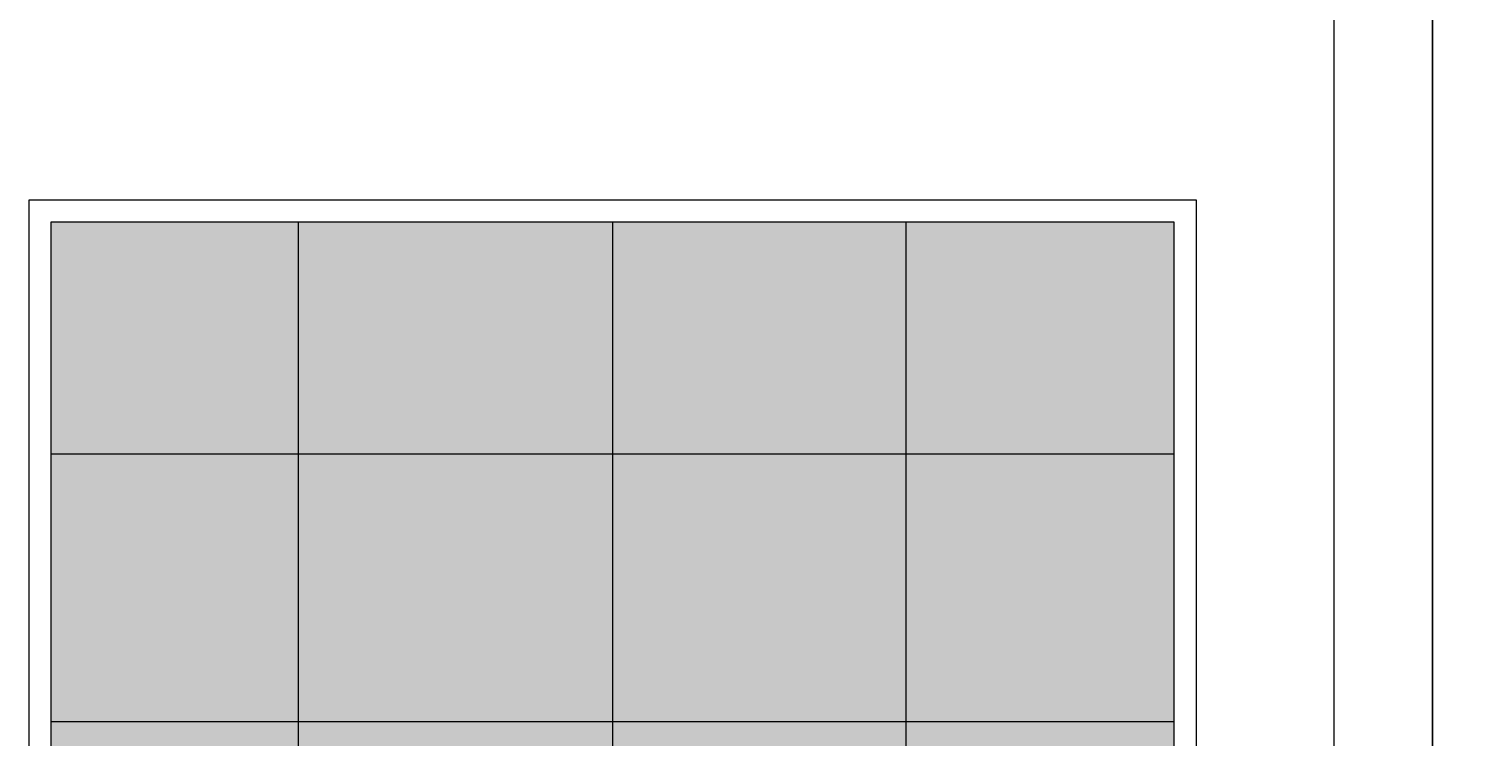
# Model space of a CAD drawing. Units: inches. Extents: x -26 to 776, y -22 to 650.
# Tile 10 of 62: x 92 to 222, y 223 to 287. Entities that reach past the tile are written whole.
import ezdxf

# ---------------------------------------------------------------- set-up
doc = ezdxf.new("R2010")
doc.units = ezdxf.units.IN
doc.header["$MEASUREMENT"] = 0
for name, color, linetype, lineweight in [('A-ANNO-DIMS', 2, 'Continuous', 18), ('A-GLAZ', 4, 'Continuous', 18), ('A-GLAZ-PATT', 9, 'Continuous', 13), ('A-WALL-TRIM', 7, 'Continuous', 18)]:
    doc.layers.add(name, color=color, linetype=linetype, lineweight=lineweight)
doc.styles.get("Standard").update_dxf_attribs({"font": 'arial.ttf'})
doc.dimstyles.get("Standard").update_dxf_attribs({"dimtxt": 0.5625, "dimasz": 0.18, "dimexe": 0.18, "dimexo": 0.0625, "dimgap": 0.09, "dimtad": 0, "dimtih": 1, "dimtoh": 1, "dimdec": 4, "dimzin": 0, "dimdsep": 46, "dimlunit": 4, "dimtxsty": 'Standard', "dimcen": 0.09, "dimadec": 0, "dimazin": 0, "dimtfac": 1, "dimtdec": 4, "dimtofl": 0, "dimtmove": 0, "dimatfit": 3, "dimfxl": 1, "dimtolj": 1, "dimtzin": 0, "dimarcsym": 0})

# ---------------------------------------------------------------- blocks, each defined once
blk = doc.blocks.new('WIN-ELEV-4X4')
for p, q in [((24.2, 97.34), (24.2, 2)), ((52.51, 97.34), (52.51, 2)), ((78.9, 97.34), (78.9, 2)), ((2, 76.47), (103.02, 76.47)), ((2, 76.47), (103.02, 76.47)), ((2, 52.37), (103.02, 52.37)), ((2, 26.9), (103.02, 26.9))]:
    blk.add_line(p, q)
for points in [[(0, 99.34), (105.02, 99.34), (105.02, 0), (0, 0)], [(2, 97.34), (103.02, 97.34), (103.02, 2), (2, 2)]]:
    blk.add_lwpolyline(points, close=True)
blk = doc.blocks.new('*D14')
at = {"layer": 'A-ANNO-DIMS', "color": 0, "lineweight": -2, "transparency": 16777216}
for p, q in [((191.62, 613.27), (-25.48, 613.27)), ((-25.3, 613.09), (-25.3, 314.75)), ((-25.3, 15.66), (-25.3, 314)), ((11.04, 15.48), (-25.48, 15.48))]:
    blk.add_line(p, q, dxfattribs=at)
at = {"layer": 'A-ANNO-DIMS', "color": 0, "transparency": 16777216}
for points in [[(-25.33, 613.09), (-25.27, 613.09), (-25.3, 613.27)], [(-25.33, 15.66), (-25.27, 15.66), (-25.3, 15.48)]]:
    blk.add_solid(points, dxfattribs=at)
at = {"layer": 'Defpoints', "color": 0, "transparency": 16777216}
for p in [(-25.3, 613.27), (191.68, 613.27), (11.11, 15.48)]:
    blk.add_point(p, dxfattribs=at)
at = {"layer": 'A-ANNO-DIMS', "color": 0, "transparency": 16777216, "insert": (-25.3, 314.38), "char_height": 0.562, "attachment_point": 5}
blk.add_mtext('\\A1;597.8', dxfattribs=at)
blk = doc.blocks.new('*D22')
at = {"layer": 'A-ANNO-DIMS', "color": 0, "lineweight": -2, "transparency": 16777216}
for p, q in [((22.89, 15.33), (22.89, 649.86)), ((23.07, 649.68), (119.19, 649.68)), ((217.77, 649.68), (121.65, 649.68)), ((217.95, 15.54), (217.95, 649.86))]:
    blk.add_line(p, q, dxfattribs=at)
at = {"layer": 'A-ANNO-DIMS', "color": 0, "transparency": 16777216}
for points in [[(23.07, 649.71), (23.07, 649.65), (22.89, 649.68)], [(217.77, 649.71), (217.77, 649.65), (217.95, 649.68)]]:
    blk.add_solid(points, dxfattribs=at)
at = {"layer": 'Defpoints', "color": 0, "transparency": 16777216}
for p in [(217.95, 649.68), (22.89, 15.27), (217.95, 15.48)]:
    blk.add_point(p, dxfattribs=at)
at = {"layer": 'A-ANNO-DIMS', "color": 0, "transparency": 16777216, "insert": (120.42, 649.68), "char_height": 0.562, "attachment_point": 5}
blk.add_mtext('\\A1;195.06', dxfattribs=at)

msp = doc.modelspace()

# ---------------------------------------------------------------- hatches: boundary and pattern name
at = {"layer": 'A-GLAZ-PATT'}
h = msp.add_hatch(dxfattribs=at)
h.set_pattern_fill('GOST_GLASS', color=256, scale=0.75)
h.set_pattern_definition([(45, (0, 0), (6.36396, 0), [3.75, -5.25]), (45, (1.591, 0), (6.36396, 0), [1.5, -7.5]), (45, (0, 1.591), (6.36396, 0), [1.5, -7.5])])
h.paths.add_polyline_path([(115.8402, 198.8773), (93.6448, 198.8773), (93.6448, 173.9734), (115.8402, 173.9734)])
h.paths.add_polyline_path([(144.1571, 198.8773), (115.8402, 198.8773), (115.8402, 173.9734), (144.1571, 173.9734)])
h.paths.add_polyline_path([(115.8402, 224.3396), (93.6448, 224.3396), (93.6448, 198.8773), (115.8402, 198.8773)])
h.paths.add_polyline_path([(144.1571, 248.4417), (115.8402, 248.4417), (115.8402, 224.3396), (144.1571, 224.3396)])
h.paths.add_polyline_path([(144.1571, 224.3396), (115.8402, 224.3396), (115.8402, 198.8773), (144.1571, 198.8773)])
h.paths.add_polyline_path([(170.5449, 224.3396), (144.1571, 224.3396), (144.1571, 198.8773), (170.5449, 198.8773)])
h.paths.add_polyline_path([(170.5449, 198.8773), (144.1571, 198.8773), (144.1571, 173.9734), (170.5449, 173.9734)])
h.paths.add_polyline_path([(194.6694, 198.8773), (170.5449, 198.8773), (170.5449, 173.9734), (194.6694, 173.9734)])
h.paths.add_polyline_path([(194.6694, 224.3396), (170.5449, 224.3396), (170.5449, 198.8773), (194.6694, 198.8773)])
h.paths.add_polyline_path([(194.6694, 248.4417), (170.5449, 248.4417), (170.5449, 224.3396), (194.6694, 224.3396)])
h.paths.add_polyline_path([(170.5449, 248.4417), (144.1571, 248.4417), (144.1571, 224.3396), (170.5449, 224.3396)])
h.paths.add_polyline_path([(144.1571, 269.3091), (115.8402, 269.3091), (115.8402, 248.4417), (144.1571, 248.4417)])
h.paths.add_polyline_path([(115.8402, 269.3091), (93.6448, 269.3091), (93.6448, 248.4417), (115.8402, 248.4417)])
h.paths.add_polyline_path([(115.8402, 248.4417), (93.6448, 248.4417), (93.6448, 224.3396), (115.8402, 224.3396)])
h.paths.add_polyline_path([(170.5449, 269.3091), (144.1571, 269.3091), (144.1571, 248.4417), (170.5449, 248.4417)])
h.paths.add_polyline_path([(194.6694, 269.3091), (170.5449, 269.3091), (170.5449, 248.4417), (194.6694, 248.4417)])
h.paths.add_polyline_path([(259.7413, 294.4171), (236.4647, 294.4171), (236.4647, 266.1888), (259.7413, 266.1888)])
h.paths.add_polyline_path([(285.0179, 294.4171), (261.7413, 294.4171), (261.7413, 266.1888), (285.0179, 266.1888)])
h.paths.add_polyline_path([(285.0179, 265.1888), (261.7413, 265.1888), (261.7413, 233.9172), (285.0179, 233.9172)])
h.paths.add_polyline_path([(259.7413, 265.1888), (236.4647, 265.1888), (236.4647, 233.9172), (259.7413, 233.9172)])
h.paths.add_polyline_path([(259.7413, 232.9172), (236.4647, 232.9172), (236.4647, 207.1741), (259.7413, 207.1741)])
h.paths.add_polyline_path([(285.0179, 232.9172), (261.7413, 232.9172), (261.7413, 207.1741), (285.0179, 207.1741)])
h.paths.add_polyline_path([(285.0179, 206.1741), (261.7413, 206.1741), (261.7413, 199.3298), (278.1134, 199.3298), (278.1134, 171.4173), (285.0179, 171.4173)])
h.paths.add_polyline_path([(259.7413, 206.1741), (236.4647, 206.1741), (236.4647, 199.3298), (259.7413, 199.3298)])
h.paths.add_polyline_path([(259.7413, 197.3298), (236.4647, 197.3298), (236.4647, 171.4173), (259.7413, 171.4173)])
h.paths.add_polyline_path([(276.1134, 197.3298), (261.7413, 197.3298), (261.7413, 171.4173), (276.1134, 171.4173)], flags=17)
h.paths.add_polyline_path([(255.8125, 548.0348), (228.5733, 548.0348), (228.5733, 528.3585), (255.8125, 528.3585)])
h.paths.add_polyline_path([(281.6181, 548.0348), (256.0792, 548.0348), (256.0792, 528.3585), (281.6181, 528.3585)])
h.paths.add_polyline_path([(308.8797, 548.0348), (281.789, 548.0348), (281.789, 528.3585), (308.8797, 528.3585)])
h.paths.add_polyline_path([(357.2724, 548.0995), (309.2457, 548.0348), (309.2457, 528.3585), (357.3034, 528.4233), (357.3034, 538.2614)])
h.paths.add_polyline_path([(259.7413, 437.1188), (236.4647, 437.1188), (236.4647, 408.8905), (259.7413, 408.8905)])
h.paths.add_polyline_path([(285.0179, 437.1188), (261.7413, 437.1188), (261.7413, 408.8905), (285.0179, 408.8905)])
h.paths.add_polyline_path([(259.7413, 407.8905), (236.4647, 407.8905), (236.4647, 376.6189), (259.7413, 376.6189)])
h.paths.add_polyline_path([(285.0179, 407.8905), (261.7413, 407.8905), (261.7413, 376.6189), (285.0179, 376.6189)])
h.paths.add_polyline_path([(285.0179, 375.6189), (261.7413, 375.6189), (261.7413, 349.8758), (285.0179, 349.8758)])
h.paths.add_polyline_path([(285.0179, 348.8758), (261.7413, 348.8758), (261.7413, 314.119), (285.0179, 314.119)])
h.paths.add_polyline_path([(259.7413, 348.8758), (236.4647, 348.8758), (236.4647, 314.119), (259.7413, 314.119)])
h.paths.add_polyline_path([(259.7413, 375.6189), (236.4647, 375.6189), (236.4647, 349.8758), (259.7413, 349.8758)])
h.paths.add_polyline_path([(194.6694, 404.1909), (170.5449, 404.1909), (170.5449, 383.3235), (194.6694, 383.3235)])
h.paths.add_polyline_path([(170.5449, 404.1909), (144.1571, 404.1909), (144.1571, 383.3235), (170.5449, 383.3235)])
h.paths.add_polyline_path([(144.1571, 404.1909), (115.8402, 404.1909), (115.8402, 383.3235), (144.1571, 383.3235)])
h.paths.add_polyline_path([(115.8402, 404.1909), (93.6448, 404.1909), (93.6448, 383.3235), (115.8402, 383.3235)])
h.paths.add_polyline_path([(115.8402, 383.3235), (93.6448, 383.3235), (93.6448, 359.2214), (115.8402, 359.2214)])
h.paths.add_polyline_path([(144.1571, 383.3235), (115.8402, 383.3235), (115.8402, 359.2214), (144.1571, 359.2214)])
h.paths.add_polyline_path([(115.8402, 359.2214), (93.6448, 359.2214), (93.6448, 333.7591), (115.8402, 333.7591)])
h.paths.add_polyline_path([(144.1571, 359.2214), (115.8402, 359.2214), (115.8402, 333.7591), (144.1571, 333.7591)])
h.paths.add_polyline_path([(115.8402, 333.7591), (93.6448, 333.7591), (93.6448, 308.8552), (115.8402, 308.8552)])
h.paths.add_polyline_path([(144.1571, 333.7591), (115.8402, 333.7591), (115.8402, 308.8552), (144.1571, 308.8552)])
h.paths.add_polyline_path([(170.5449, 333.7591), (144.1571, 333.7591), (144.1571, 308.8552), (170.5449, 308.8552)])
h.paths.add_polyline_path([(170.5449, 359.2214), (144.1571, 359.2214), (144.1571, 333.7591), (170.5449, 333.7591)])
h.paths.add_polyline_path([(170.5449, 383.3235), (144.1571, 383.3235), (144.1571, 359.2214), (170.5449, 359.2214)])
h.paths.add_polyline_path([(194.6694, 383.3235), (170.5449, 383.3235), (170.5449, 359.2214), (194.6694, 359.2214)])
h.paths.add_polyline_path([(194.6694, 359.2214), (170.5449, 359.2214), (170.5449, 333.7591), (194.6694, 333.7591)])
h.paths.add_polyline_path([(194.6694, 333.7591), (170.5449, 333.7591), (170.5449, 308.8552), (194.6694, 308.8552)])

# ---------------------------------------------------------------- linework, layer by layer
at = {"layer": 'A-WALL-TRIM'}
msp.add_lwpolyline([(82.134, 159.4824), (209.091, 159.4824), (209.091, 420.2783), (82.134, 420.2783)], close=True, dxfattribs=at)

# ---------------------------------------------------------------- block references
at = {"layer": 'A-GLAZ'}
msp.add_blockref('WIN-ELEV-4X4', (91.645, 171.9733), dxfattribs=at)

# ---------------------------------------------------------------- dimensions: what is measured, and where the dimension line sits
at = {"layer": 'A-ANNO-DIMS'}
dim = msp.add_linear_dim(base=(217.9529, 649.6763), p1=(22.8891, 15.2701), p2=(217.9529, 15.4824), dimstyle='Standard', override={"dimdec": 2, "dimlfac": 1, "dimrnd": 0, "dimzin": 0, "dimdsep": 46, "dimlunit": 2}, dxfattribs=at)
dim.commit()
dim.dimension.update_dxf_attribs({"geometry": '*D22', "text_midpoint": (120.421, 649.6763)})
dim = msp.add_linear_dim(base=(-25.2976, 613.2713), p1=(11.1074, 15.4824), p2=(191.6782, 613.2713), angle=90, dimstyle='Standard', override={"dimdec": 1, "dimlfac": 1, "dimrnd": 0, "dimzin": 0, "dimdsep": 46, "dimlunit": 2}, dxfattribs=at)
dim.commit()
dim.dimension.update_dxf_attribs({"geometry": '*D14', "text_midpoint": (-25.2976, 314.3769)})

doc.saveas('drawing.dxf')
